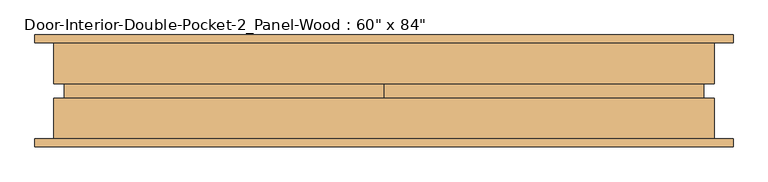
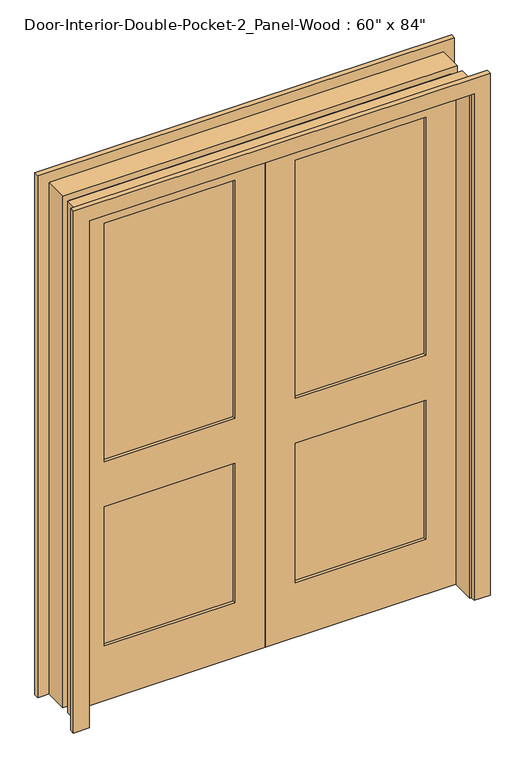
"""IFC4 building model written with IfcOpenShell, lengths in millimetres: door geometry."""

from ifc_helpers import new_model, si_unit, frame, origin, place, context, project, spatial, polyline, outline, extrude, source, transform, mapped, element, save


def door_7a66d0d1(model_context):
    return source(origin(), model_context, "Body", "SweptSolid", [
        extrude(outline(polyline([(0.0, 768.35), (0.0, 831.85), (2203.45, 831.85), (2203.45, -831.85), (0.0, -831.85), (0.0, -768.35), (2139.95, -768.35), (2139.95, 768.35), (0.0, 768.35)])), frame((0.0, 114.3, 0.0), z_axis=(0.0, 1.0, 0.0), x_axis=(0.0, 0.0, 1.0)), (0.0, 0.0, 1.0), 19.05),
        extrude(outline(polyline([(0.0, 768.35), (0.0, 831.85), (2203.45, 831.85), (2203.45, -831.85), (0.0, -831.85), (0.0, -768.35), (2139.95, -768.35), (2139.95, 768.35), (0.0, 768.35)])), frame((0.0, -133.35, 0.0), z_axis=(0.0, 1.0, 0.0), x_axis=(0.0, 0.0, 1.0)), (0.0, 0.0, 1.0), 19.05),
        extrude(outline(polyline([(2133.6, 0.0), (0.0, 0.0), (0.0, 762.0), (2133.6, 762.0), (2133.6, 0.0)]), holes=[polyline([(2014.5375, 120.65), (2014.5375, 641.35), (1009.65, 641.35), (1009.65, 120.65), (2014.5375, 120.65)]), polyline([(819.15, 120.65), (819.15, 641.35), (231.775, 641.35), (231.775, 120.65), (819.15, 120.65)])]), frame((0.0, -17.4625, 0.0), z_axis=(0.0, 1.0, 0.0), x_axis=(0.0, 0.0, 1.0)), (0.0, 0.0, 1.0), 34.925),
        extrude(outline(polyline([(641.35, -5.8208333), (120.65, -5.8208333), (120.65, 5.8208333), (641.35, 5.8208333), (641.35, -5.8208333)])), frame((0.0, 0.0, 1009.65), z_axis=(0.0, 0.0, 1.0), x_axis=(1.0, 0.0, 0.0)), (0.0, 0.0, 1.0), 1004.8875),
        extrude(outline(polyline([(641.35, -5.8208333), (120.65, -5.8208333), (120.65, 5.8208333), (641.35, 5.8208333), (641.35, -5.8208333)])), frame((0.0, 0.0, 231.775), z_axis=(0.0, 0.0, 1.0), x_axis=(1.0, 0.0, 0.0)), (0.0, 0.0, 1.0), 587.375),
        extrude(outline(polyline([(0.0, 787.4), (2159.0, 787.4), (2159.0, -787.4), (0.0, -787.4), (0.0, -762.0), (2133.6, -762.0), (2133.6, 762.0), (0.0, 762.0), (0.0, 787.4)])), frame((0.0, 17.4625, 0.0), z_axis=(0.0, 1.0, 0.0), x_axis=(0.0, 0.0, 1.0)), (0.0, 0.0, 1.0), 96.8375),
        extrude(outline(polyline([(0.0, 787.4), (2159.0, 787.4), (2159.0, -787.4), (0.0, -787.4), (0.0, -762.0), (2133.6, -762.0), (2133.6, 762.0), (0.0, 762.0), (0.0, 787.4)])), frame((0.0, -114.3, 0.0), z_axis=(0.0, 1.0, 0.0), x_axis=(0.0, 0.0, 1.0)), (0.0, 0.0, 1.0), 96.8375),
        extrude(outline(polyline([(2133.6, -762.0), (0.0, -762.0), (0.0, 0.0), (2133.6, 0.0), (2133.6, -762.0)]), holes=[polyline([(2014.5375, -641.35), (2014.5375, -120.65), (1009.65, -120.65), (1009.65, -641.35), (2014.5375, -641.35)]), polyline([(819.15, -641.35), (819.15, -120.65), (231.775, -120.65), (231.775, -641.35), (819.15, -641.35)])]), frame((0.0, -17.4625, 0.0), z_axis=(0.0, 1.0, 0.0), x_axis=(0.0, 0.0, 1.0)), (0.0, 0.0, 1.0), 34.925),
        extrude(outline(polyline([(-120.65, -5.8208333), (-641.35, -5.8208333), (-641.35, 5.8208333), (-120.65, 5.8208333), (-120.65, -5.8208333)])), frame((0.0, 0.0, 1009.65), z_axis=(0.0, 0.0, 1.0), x_axis=(1.0, 0.0, 0.0)), (0.0, 0.0, 1.0), 1004.8875),
        extrude(outline(polyline([(-120.65, -5.8208333), (-641.35, -5.8208333), (-641.35, 5.8208333), (-120.65, 5.8208333), (-120.65, -5.8208333)])), frame((0.0, 0.0, 231.775), z_axis=(0.0, 0.0, 1.0), x_axis=(1.0, 0.0, 0.0)), (0.0, 0.0, 1.0), 587.375),
    ])


if __name__ == "__main__":
    model = new_model("IFC4")
    model_context = context("Model", 3, world=origin())
    ifc_project = project(units=[si_unit("LENGTHUNIT", "METRE", prefix="MILLI")], contexts=[model_context])
    site = spatial("IfcSite", under=ifc_project)
    building = spatial("IfcBuilding", under=site)
    placement = place(None, origin())
    door_shape = door_7a66d0d1(model_context)
    element("IfcDoor", 1, ObjectType="Door-Interior-Double-Pocket-2_Panel-Wood : 60\" x 84\"", at=placement, inside=building, context=model_context, shape_type="MappedRepresentation", body=[
        mapped(door_shape, transform((0.0, 0.0, 0.0), x_axis=(1.0, 0.0, 0.0), y_axis=(0.0, 1.0, 0.0), z_axis=(0.0, 0.0, 1.0))),
    ])
    save(model, "model.ifc")

# Revit data of these elements
# Type "Door-Interior-Double-Pocket-2_Panel-Wood : 60\" x 84\""
#   Type Mark = "8"
#   Assembly Code = "C1020300"
#   Analytic Construction = "Wooden"
#   Top Rail = 0' - 4 11/16"
#   Thickness = 0' - 1 3/8"
#   Thermal Resistance (R) = 2.5876 (h·ft²·°F)/BTU
#   Stiles = 0' - 4 3/4"
#   Rough Width = 10' - 2"
#   Rough Height = 7' - 4 1/2"
#   Panel Width = 2' - 6"
#   Lock Rail = 0' - 7 1/2"
#   Location [instance default] = 2' - 7"
#   Height = 7' - 0"
#   Width = 5' - 0"
#   Heat Transfer Coefficient (U) = 0.3865 BTU/(h·ft²·°F)
#   Bottom Rail = 0' - 9 1/8"
#   Panel Open [instance default] = no
#   Trim Material = Cherry
#   Panel Material = Cherry
#   Frame Material = Cherry
#   Visual Light Transmittance = 0
#   Solar Heat Gain Coefficient = 0
#   Wall Closure = (empty or 0)
#   Function = (empty or 0)
# Element 1 (IfcDoor, "Door-Interior-Double-Pocket-2_Panel-Wood : 60\" x 84\"")
#   Materials on its faces: "Cherry"
# Materials
#   "Cherry": class "Wood", colour RGB 226 177 128, transparency 0, Description = "Prunus Serotina", Cost = 0
